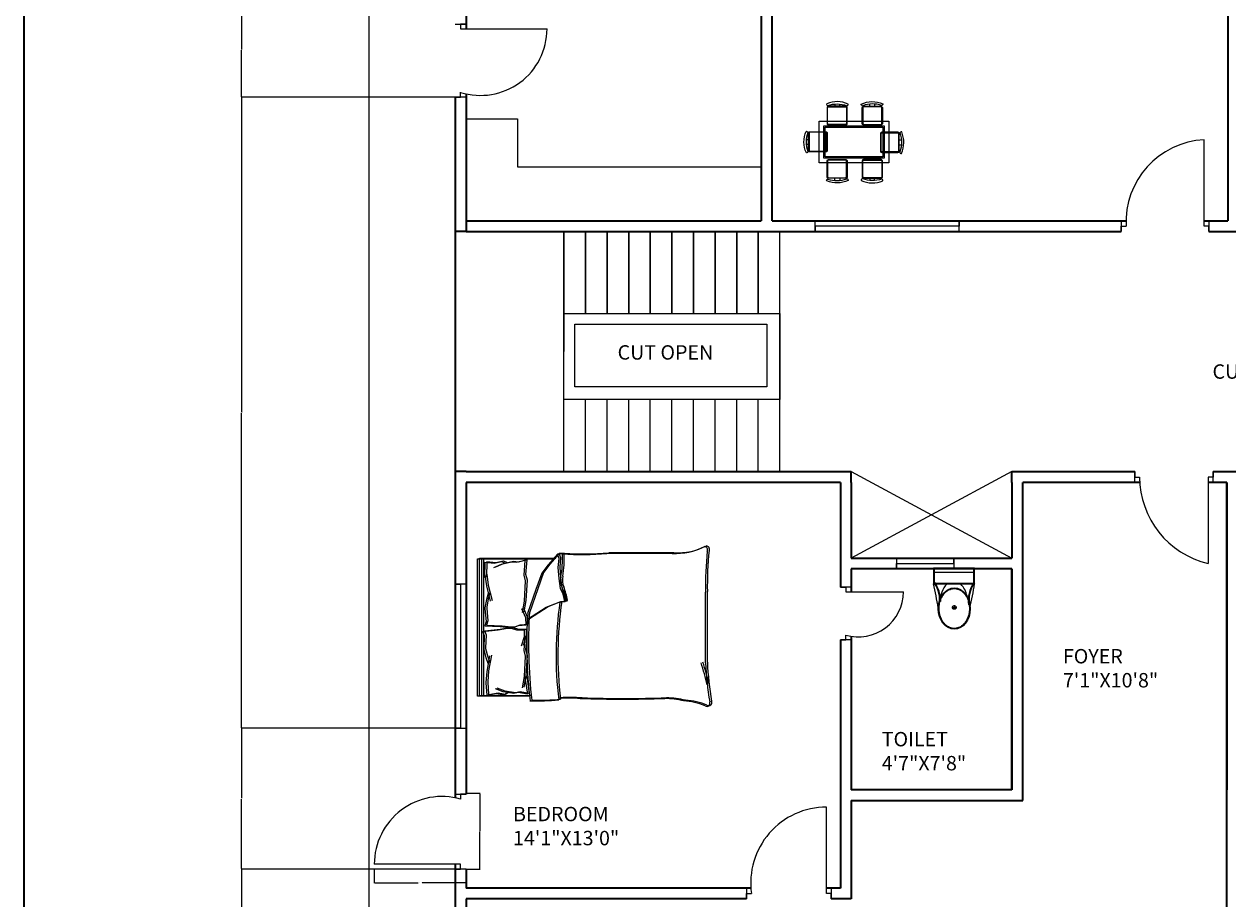
# Model space of a CAD drawing. Units: inches. Extents: x 1520 to 3401, y 1570 to 3432.
# Tile 4 of 15: x 1520 to 2022, y 2061 to 2425. Entities that reach past the tile are written whole.
import ezdxf

# ---------------------------------------------------------------- set-up
doc = ezdxf.new("R2010")
doc.units = ezdxf.units.IN
for name, color, linetype, lineweight in [('A-ANNO-DIMS', 2, 'Continuous', 18), ('A-ANNO-TTLB', 7, 'Continuous', 35), ('A-AREA-IDEN', 7, 'Continuous', 18), ('A-DOOR', 3, 'Continuous', 18), ('A-FLOR-CASE', 8, 'Continuous', 18), ('A-FLOR-EDGE', 7, 'Continuous', 25), ('A-FLOR-FIXT', 9, 'Continuous', 18), ('A-FLOR-OPEN', 8, 'Continuous', 13), ('A-FLOR-STRS', 2, 'Continuous', 18), ('A-FURN', 8, 'Continuous', 13), ('A-GLAZ', 4, 'Continuous', 18), ('A-WALL', 7, 'Continuous', 35)]:
    doc.layers.add(name, color=color, linetype=linetype, lineweight=lineweight)
doc.styles.get("Standard").update_dxf_attribs({"font": 'arial.ttf'})
doc.dimstyles.get("Standard").update_dxf_attribs({"dimtxt": 0.18, "dimasz": 0.18, "dimexe": 0.18, "dimexo": 0.0625, "dimgap": 0.09, "dimtad": 0, "dimtih": 1, "dimtoh": 1, "dimdec": 4, "dimzin": 0, "dimdsep": 46, "dimtxsty": 'Standard', "dimcen": 0.09, "dimadec": 0, "dimazin": 0, "dimtfac": 1, "dimtdec": 4, "dimtofl": 0, "dimtmove": 0, "dimatfit": 3, "dimfxl": 1, "dimtolj": 1, "dimtzin": 0, "dimarcsym": 0})

# ---------------------------------------------------------------- blocks, each defined once
blk = doc.blocks.new('A$C31115884')
for p, q in [((283, 498), (223, 498)), ((258, 466), (258, 523)), ((0, 200), (0, 0)), ((520, 200), (0, 200)), ((10, 190), (10, 10)), ((510, 190), (10, 190)), ((510, 10), (510, 190)), ((520, 0), (520, 200)), ((510, 54), (0, 54)), ((10, 10), (510, 10)), ((0, 0), (520, 0))]:
    blk.add_line(p, q)
blk.add_circle((256, 496), 23.6)
for centre, radius, start, end in [((2778, -205), 2807, 165.4549, 171.7133), ((-295, 403), 365, 324.2091, 9.3499), ((-295, 403), 375, 324.2091, 9.3499), ((806, 403), 365, 170.6501, 215.7909), ((3237, 905), 2807, 188.2867, 194.5451), ((384, 406), 293, 190.2774, 224.1564), ((139, 406), 293, 315.8436, 2.6563), ((806, 403), 375, 179.2036, 215.7909)]:
    blk.add_arc(centre, radius, start, end)
blk.add_ellipse((256, 510), major_axis=(0, -261), ratio=0.772727)
blk.add_open_spline([(256, 259), (263, 259), (270, 260), (288, 262), (299, 265), (320, 273), (330, 278), (350, 291), (360, 299), (378, 316), (386, 326), (402, 347), (409, 358), (421, 383), (427, 395), (436, 422), (440, 436), (445, 465), (447, 480), (448, 509), (448, 524), (445, 553), (443, 568), (436, 596), (432, 610), (422, 636), (416, 649), (402, 672), (395, 683), (379, 703), (370, 712), (351, 728), (341, 735), (321, 746), (310, 751), (289, 757), (278, 759), (256, 761), (245, 761), (223, 757), (212, 754), (191, 746), (181, 741), (161, 728), (151, 720), (133, 703), (125, 693), (110, 672), (103, 660), (90, 636), (85, 623), (76, 596), (72, 582), (67, 553), (66, 538), (64, 509), (65, 494), (68, 465), (70, 450), (77, 422), (81, 408), (91, 382), (97, 370), (111, 346), (118, 335), (135, 316), (144, 307), (162, 291), (172, 284), (193, 273), (203, 269), (225, 262), (236, 260), (250, 259), (253, 259), (256, 259)], degree=3, knots=[0, 0, 0, 0, 0.110105, 0.110105, 0.285049, 0.285049, 0.459994, 0.459994, 0.634938, 0.634938, 0.809882, 0.809882, 0.984827, 0.984827, 1.159771, 1.159771, 1.334715, 1.334715, 1.50966, 1.50966, 1.684604, 1.684604, 1.859549, 1.859549, 2.034493, 2.034493, 2.209437, 2.209437, 2.384382, 2.384382, 2.559326, 2.559326, 2.73427, 2.73427, 2.909215, 2.909215, 3.084159, 3.084159, 3.259103, 3.259103, 3.434048, 3.434048, 3.608992, 3.608992, 3.783936, 3.783936, 3.958881, 3.958881, 4.133825, 4.133825, 4.30877, 4.30877, 4.483714, 4.483714, 4.658658, 4.658658, 4.833603, 4.833603, 5.008547, 5.008547, 5.183491, 5.183491, 5.358436, 5.358436, 5.53338, 5.53338, 5.708324, 5.708324, 5.883269, 5.883269, 6.058213, 6.058213, 6.233158, 6.233158, 6.283185, 6.283185, 6.283185, 6.283185])
blk = doc.blocks.new('DOOR-SWING-36-09')
for p, q in [((34.55, 2.25), (34.55, 38.25)), ((0, 4.5), (0, 0)), ((0, 0), (0, 2.25)), ((0, 2.25), (2, 2.25)), ((36.55, 2.25), (34.55, 2.25)), ((36.55, 4.5), (36.55, 0)), ((36.55, 0), (36.55, 2.25))]:
    blk.add_line(p, q)
blk.add_arc((36.37, 3.88), 34.41, 93.0408, 182.7237)
blk = doc.blocks.new('DOOR-SWING-24-14')
for p, q in [((4.5, 21.95), (0, 21.95)), ((0, 21.95), (2.25, 21.95)), ((2.25, 21.95), (2.25, 19.95)), ((2.25, 19.95), (26.25, 19.95)), ((4.5, 0), (0, 0)), ((0, 0), (2.25, 0)), ((2.25, 0), (2.25, 2))]:
    blk.add_line(p, q)
blk.add_arc((7.54, 19.95), 18.71, 253.5847, 0)
blk = doc.blocks.new('DOOR-SWING-36-15')
for p, q in [((33.3, 2.25), (33.3, 38.25)), ((0, 4.5), (0, 0)), ((0, 0), (0, 2.25)), ((0, 2.25), (2, 2.25)), ((35.3, 2.25), (33.3, 2.25)), ((35.3, 4.5), (35.3, 0)), ((35.3, 0), (35.3, 2.25))]:
    blk.add_line(p, q)
blk.add_arc((33.3, 6.65), 31.6, 90, 187.995)
blk = doc.blocks.new('DOOR-SWING-36-17')
for p, q in [((0, 33.75), (0, 38.25)), ((0, 38.25), (0, 36)), ((0, 36), (2, 36)), ((32.63, 36), (30.63, 36)), ((30.63, 36), (30.63, 0)), ((32.63, 33.75), (32.63, 38.25)), ((32.63, 38.25), (32.63, 36))]:
    blk.add_line(p, q)
blk.add_arc((38.95, 36), 36.95, 180, 256.9796)
blk = doc.blocks.new('DOOR-SWING-36-24')
for p, q in [((0, 30.42), (4.5, 30.42)), ((4.5, 30.42), (2.25, 30.42)), ((2.25, 30.42), (2.25, 28.42)), ((2.25, 28.42), (38.25, 28.42)), ((4.5, 0), (0, 0)), ((0, 0), (2.25, 0)), ((2.25, 0), (2.25, 2))]:
    blk.add_line(p, q)
blk.add_arc((10.55, 28.42), 27.7, 252.5577, 0)
blk = doc.blocks.new('DOOR-SWING-36-25')
for p, q in [((33.75, 31.15), (38.25, 31.15)), ((38.25, 31.15), (36, 31.15)), ((36, 31.15), (36, 29.15)), ((36, 2), (0, 2)), ((38.25, 0), (33.75, 0)), ((33.75, 0), (36, 0)), ((36, 0), (36, 2))]:
    blk.add_line(p, q)
blk.add_arc((28.23, 2), 28.23, 74.0345, 180)
blk = doc.blocks.new('WIN-PLAN-24-01')
for p, q in [((0, 4.5), (0, 0)), ((0, 0), (0, 2.25)), ((0, 2.25), (24, 2.25)), ((24, 2.25), (24, 4.5)), ((24, 4.5), (24, 0))]:
    blk.add_line(p, q)
blk = doc.blocks.new('WIN-PLAN-60-02')
for p, q in [((4.5, 60), (0, 60)), ((0, 60), (2.25, 60)), ((2.25, 60), (2.25, 0)), ((4.5, 0), (0, 0)), ((2.25, 0), (4.5, 0))]:
    blk.add_line(p, q)
blk = doc.blocks.new('WIN-PLAN-60-03')
for p, q in [((0, 2.25), (0, 4.5)), ((0, 4.5), (0, 0)), ((60, 2.25), (0, 2.25)), ((60, 0), (60, 4.5)), ((60, 4.5), (60, 2.25))]:
    blk.add_line(p, q)
blk = doc.blocks.new('BED-DOUBLE')
for p, q in [((4.17, 75.93), (4.17, 97.64)), ((4.17, 97.64), (61.46, 97.64)), ((4.17, 95.8), (61.46, 95.8)), ((4.44, 75.16), (4.44, 96.87)), ((4.44, 96.87), (61.73, 96.87)), ((29.42, 94.7), (31.15, 95.4)), ((31.15, 95.4), (31.84, 88.98)), ((61.46, 97.64), (61.46, 65.74)), ((61.73, 96.87), (61.73, 64.97)), ((4.44, 95.03), (61.73, 95.03)), ((4.67, 93.64), (9.81, 94.03)), ((4.67, 93.66), (5.36, 89.85)), ((4.94, 92.9), (5.64, 89.08)), ((4.95, 92.87), (10.08, 93.27)), ((9.81, 94.03), (9.93, 94.01)), ((9.93, 94.01), (14.52, 93.66)), ((10.08, 93.27), (10.21, 93.24)), ((10.21, 93.24), (14.79, 92.9)), ((14.52, 93.66), (21.1, 92.45)), ((14.79, 92.9), (21.38, 91.68)), ((17.81, 93.14), (20.24, 94.01)), ((18.08, 92.38), (20.51, 93.24)), ((20.24, 94.01), (23.7, 94.88)), ((20.51, 93.24), (23.98, 94.11)), ((23.7, 94.88), (24.09, 94.88)), ((23.98, 94.11), (24.36, 94.11)), ((24.09, 94.88), (29.42, 94.7)), ((24.36, 94.11), (29.69, 93.94)), ((29.69, 93.94), (31.42, 94.63)), ((31.42, 94.63), (32.12, 88.22)), ((33.54, 94.65), (33.25, 88.21)), ((33.81, 93.88), (33.52, 87.44)), ((35.31, 94.07), (33.54, 94.65)), ((35.59, 93.3), (33.81, 93.88)), ((40.62, 94.57), (35.31, 94.07)), ((40.9, 93.81), (35.59, 93.3)), ((41.01, 94.6), (40.62, 94.57)), ((41.28, 93.83), (40.9, 93.81)), ((44.52, 93.95), (41.01, 94.6)), ((44.79, 93.18), (41.28, 93.83)), ((50.25, 93.96), (43.75, 92.34)), ((50.52, 93.19), (44.03, 91.57)), ((47, 93.23), (44.52, 93.95)), ((47.27, 92.47), (44.79, 93.18)), ((54.8, 94.59), (50.25, 93.96)), ((55.08, 93.82), (50.52, 93.19)), ((60.08, 94.57), (53.6, 94.69)), ((53.6, 94.69), (54.8, 94.59)), ((60.35, 93.81), (53.87, 93.92)), ((53.87, 93.92), (55.08, 93.82)), ((59.12, 87.74), (57.7, 90.95)), ((60.08, 94.57), (59.62, 90.72)), ((59.62, 90.72), (60.34, 87.64)), ((60.35, 93.81), (59.9, 89.96)), ((5.36, 89.85), (4.84, 86.73)), ((4.84, 86.73), (5.54, 85.52)), ((5.64, 89.08), (5.12, 85.96)), ((5.12, 85.96), (5.81, 84.75)), ((5.36, 82.57), (6.06, 86.9)), ((5.64, 81.8), (6.33, 86.14)), ((6.06, 86.9), (7.27, 90.2)), ((6.33, 86.14), (7.54, 89.43)), ((31.84, 88.98), (32.54, 85.17)), ((32.12, 88.22), (32.81, 84.4)), ((33.25, 88.21), (32.79, 84.36)), ((33.52, 87.44), (33.07, 83.59)), ((59.39, 86.97), (57.97, 90.18)), ((60.08, 83.46), (59.12, 87.74)), ((60.35, 82.69), (59.39, 86.97)), ((60.34, 87.64), (59.72, 86.39)), ((59.9, 89.96), (60.61, 86.88)), ((60.61, 86.88), (59.99, 85.62)), ((5.02, 76.85), (5.71, 80.66)), ((5.71, 80.66), (5.36, 82.57)), ((5.98, 79.9), (5.64, 81.8)), ((32.54, 83.61), (31.84, 81.36)), ((31.84, 81.36), (31.84, 78.14)), ((32.81, 82.84), (32.12, 80.59)), ((32.12, 80.59), (32.12, 77.37)), ((32.54, 85.17), (32.54, 83.61)), ((32.79, 84.36), (32.89, 82.8)), ((32.81, 84.4), (32.81, 82.84)), ((32.89, 82.8), (33.72, 80.59)), ((33.07, 83.59), (33.17, 82.03)), ((33.17, 82.03), (34, 79.83)), ((33.72, 80.59), (33.93, 77.39)), ((59.85, 81.53), (60.08, 83.46)), ((60.78, 77.77), (59.85, 81.53)), ((60.12, 80.77), (60.35, 82.69)), ((61.05, 77), (60.12, 80.77)), ((11.13, 77.72), (5.02, 76.85)), ((5.29, 76.08), (5.98, 79.9)), ((11.4, 76.95), (5.29, 76.08)), ((7.65, 78.9), (12.48, 78.1)), ((7.92, 78.14), (12.76, 77.34)), ((12.48, 78.1), (11.13, 77.72)), ((12.76, 77.34), (11.4, 76.95)), ((12.48, 78.1), (20.89, 77.59)), ((12.76, 77.34), (21.16, 76.82)), ((20.89, 77.59), (23.24, 78.25)), ((21.16, 76.82), (23.51, 77.49)), ((23.24, 78.25), (29.39, 77.77)), ((23.51, 77.49), (29.67, 77)), ((28.9, 78.14), (25.13, 79.45)), ((29.17, 77.37), (25.4, 78.68)), ((31.84, 78.14), (28.9, 78.14)), ((32.12, 77.37), (29.17, 77.37)), ((33.93, 77.39), (36.87, 77.57)), ((34, 79.83), (34.2, 76.62)), ((34.2, 76.62), (37.14, 76.8)), ((36.28, 76.8), (41.3, 69.01)), ((36.55, 76.03), (41.57, 68.25)), ((36.87, 77.57), (40.55, 79.11)), ((37.14, 76.8), (40.82, 78.34)), ((48.73, 73.28), (38.73, 76.8)), ((49, 72.52), (39, 76.03)), ((39.04, 78.9), (43.87, 78.1)), ((39.31, 78.14), (44.15, 77.34)), ((43.87, 78.1), (52.28, 77.59)), ((44.15, 77.34), (52.55, 76.82)), ((52.28, 77.59), (54.63, 78.25)), ((52.55, 76.82), (54.9, 77.49)), ((54.63, 78.25), (60.78, 77.77)), ((54.9, 77.49), (61.05, 77)), ((55.41, 70.87), (48.73, 73.28)), ((55.69, 70.1), (49, 72.52)), ((58.94, 68.27), (55.41, 70.87)), ((41.3, 69.01), (43.34, 63.63)), ((41.57, 68.25), (43.62, 62.87)), ((59.21, 67.51), (55.69, 70.1)), ((63.38, 64.38), (58.94, 68.27)), ((63.66, 63.61), (59.21, 67.51)), ((43.34, 63.63), (43.71, 61.22)), ((43.62, 62.87), (43.99, 60.45)), ((43.71, 61.22), (46.68, 61.96)), ((43.99, 60.45), (46.96, 61.2)), ((46.68, 61.96), (49.1, 63.08)), ((46.96, 61.2), (49.37, 62.31)), ((49.1, 63.08), (53.18, 63.63)), ((49.37, 62.31), (53.46, 62.87)), ((53.18, 63.63), (57.82, 64)), ((53.46, 62.87), (58.1, 63.24)), ((57.82, 64), (61.54, 63.63)), ((58.1, 63.24), (61.81, 62.87)), ((61.54, 63.63), (63.38, 64.38)), ((61.81, 62.87), (63.66, 63.61)), ((63.48, 62.28), (63.38, 64.38, 4.64)), ((63.75, 61.52), (63.66, 63.61, 4.64)), ((18.06, 2.64), (47.57, 2.64)), ((18.33, 1.87), (47.84, 1.87))]:
    blk.add_line(p, q)
for centre, radius, start, end in [((102.1, 73.55), 99.87, 178.7218, 185.604), ((25.61, -120.62), 197.77, 86.0865, 96.7821), ((25.88, -121.38), 197.77, 86.0865, 96.7821), ((102.37, 72.78), 99.87, 178.7218, 185.604), ((21.29, -89.76), 154.68, 81.7845, 96.9006), ((21.56, -90.53), 154.68, 81.7845, 96.9006), ((-200.58, 60.27), 203.94, 358.4762, 1.0082), ((-200.3, 59.5), 203.94, 358.4762, 1.0082), ((43.92, 61.15), 0.221, 160.2464, 271.1377), ((37.35, 95.86), 35.55, 280.6617, 289.8806), ((44.2, 60.38), 0.221, 160.2464, 271.1377), ((37.62, 95.1), 35.55, 280.6617, 289.8806), ((52.44, 55.6), 7.46, 78.6608, 113.7384), ((52.72, 54.83), 7.46, 78.6608, 113.7384), ((61.53, 105.62), 43.38, 259.8763, 272.5657), ((61.81, 104.85), 43.38, 259.8763, 272.5657), ((218.51, 54.1), 155.25, 176.9791, 183.8365), ((218.79, 53.34), 155.25, 176.9791, 183.8365), ((581.23, 36.96), 578.22, 178.22771, 181.71854), ((581.51, 36.19), 578.22, 178.22771, 181.71854), ((-5405.34, 16.33), 5469.02, 0.00217, 0.28689), ((-5405.07, 15.56), 5469.02, 0.00217, 0.28689), ((-32.25, 20.29), 35.53, 346.0648, 358.9113), ((-31.97, 19.53), 35.53, 346.0648, 358.9113), ((91.3, 15.32), 27.65, 177.4714, 206.4681), ((91.58, 14.55), 27.65, 177.4714, 206.4681), ((-25.97, 13.39), 28.25, 337.9751, 356.652), ((-25.69, 12.62), 28.25, 337.9751, 356.652), ((1.3, 2.07), 1.31, 146.1736, 293.4781), ((1.58, 1.3), 1.31, 146.1736, 293.4781), ((25.69, -143.14), 145.97, 92.9958, 99.4091), ((25.96, -143.9), 145.97, 92.9958, 99.4091), ((-20.65, 126.07), 127.63, 283.3832, 287.7053), ((-20.37, 125.3), 127.63, 283.3832, 287.7053), ((49.34, -156.85), 159.5, 84.4998, 90.6351), ((49.61, -157.62), 159.5, 84.4998, 90.6351), ((65.23, 3.08), 1.32, 242.6588, 356.02), ((65.5, 2.32), 1.32, 242.6588, 356.02)]:
    blk.add_arc(centre, radius, start, end)
blk = doc.blocks.new('KITCHEN-COUNTER-04')
for p, q in [((0, 19.94), (21.46, 19.94)), ((21.46, 19.94), (21.46, 0)), ((21.46, 0), (123, 0)), ((123, 0), (123, 0))]:
    blk.add_line(p, q)
blk = doc.blocks.new('DINING-SET-6-SEAT')
for points in [[(9.94, 32.23, -0.175809), (17.84, 32.17, 0.578392), (18.44, 32.83, 0.214524), (9.52, 32.95, 0.552014), (9.94, 32.23, -0.065079)], [(17.51, 31.92), (10.17, 31.92, 0.414214), (9.66, 31.4), (9.66, 24.66, 0.414214), (10.17, 24.14), (17.51, 24.14, 0.414214), (18.02, 24.66), (18.02, 31.4, 0.414214), (17.51, 31.92)], [(14.93, 31.92), (14.93, 32.84, -0.064759)], [(24.5, 32.17, -0.578392), (23.9, 32.83, -0.214524), (32.82, 32.95, -0.552014), (32.4, 32.23, 0.175809), (24.5, 32.17)], [(32.17, 31.92, -0.414214), (32.68, 31.4), (32.68, 24.66, -0.414214), (32.17, 24.14), (24.83, 24.14, -0.414214), (24.32, 24.66), (24.32, 31.4, -0.414214), (24.83, 31.92), (32.17, 31.92)], [(27.41, 31.92), (27.41, 32.84, 0.064759)], [(1.67, 13.15, -0.578392), (1.02, 12.55, -0.214524), (0.9, 21.47, -0.552014), (1.61, 21.05, 0.175809), (1.67, 13.15)], [(1.93, 20.82, -0.414214), (2.45, 21.33), (9.19, 21.33, -0.414214), (9.7, 20.82), (9.7, 13.49, -0.414214), (9.19, 12.97), (2.45, 12.97, -0.414214), (1.93, 13.49), (1.93, 20.82)], [(39.71, 20.57, 0.414214), (39.19, 21.08), (32.45, 21.08, 0.414214), (31.94, 20.57), (31.94, 13.23, 0.414214), (32.45, 12.72), (39.19, 12.72, 0.414214), (39.71, 13.23), (39.71, 20.57)], [(40.02, 20.8, -0.175809), (39.96, 12.9, 0.578392), (40.62, 12.3, 0.214524), (40.74, 21.22, 0.552014), (40.02, 20.8, -0.065079)], [(1.93, 16.06), (1, 16.06, 0.064759)], [(39.71, 15.81), (40.63, 15.81, -0.064759)], [(17.51, 1.93), (10.17, 1.93, -0.414214), (9.66, 2.45), (9.66, 9.19, -0.414214), (10.17, 9.7), (17.51, 9.7, -0.414214), (18.02, 9.19), (18.02, 2.45, -0.414214), (17.51, 1.93)], [(32.17, 1.93, 0.414214), (32.68, 2.45), (32.68, 9.19, 0.414214), (32.17, 9.7), (24.83, 9.7, 0.414214), (24.32, 9.19), (24.32, 2.45, 0.414214), (24.83, 1.93), (32.17, 1.93)], [(17.84, 1.67, -0.578392), (18.44, 1.02, -0.214524), (9.52, 0.9, -0.552014), (9.94, 1.61, 0.175809), (17.84, 1.67)], [(14.93, 1.93), (14.93, 1, 0.064759)], [(32.4, 1.61, -0.175809), (24.5, 1.67, 0.578392), (23.9, 1.02, 0.214524), (32.82, 0.9, 0.552014), (32.4, 1.61, -0.065079)], [(27.41, 1.93), (27.41, 1, -0.064759)]]:
    blk.add_lwpolyline(points, format="xyb")
for points in [[(10.18, 31.68), (17.28, 31.68, -0.414214), (17.79, 31.17), (17.79, 24.89, -0.414214), (17.28, 24.37), (10.18, 24.37, -0.512069), (9.89, 24.89), (9.89, 31.17, -0.512069)], [(32.16, 31.68), (25.06, 31.68, 0.414214), (24.55, 31.17), (24.55, 24.89, 0.414214), (25.06, 24.37), (32.16, 24.37, 0.512069), (32.45, 24.89), (32.45, 31.17, 0.512069)], [(2.16, 20.82), (2.16, 13.72, 0.414214), (2.68, 13.2), (8.96, 13.2, 0.414214), (9.47, 13.72), (9.47, 20.82, 0.512069), (8.96, 21.1), (2.68, 21.1, 0.512069)], [(39.48, 20.57), (39.48, 13.47, -0.414214), (38.96, 12.95), (32.68, 12.95, -0.414214), (32.17, 13.47), (32.17, 20.57, -0.512069), (32.68, 20.85), (38.96, 20.85, -0.512069)], [(10.18, 2.16), (17.28, 2.16, 0.414214), (17.79, 2.68), (17.79, 8.96, 0.414214), (17.28, 9.47), (10.18, 9.47, 0.512069), (9.89, 8.96), (9.89, 2.68, 0.512069)], [(32.16, 2.16), (25.06, 2.16, -0.414214), (24.55, 2.68), (24.55, 8.96, -0.414214), (25.06, 9.47), (32.16, 9.47, -0.512069), (32.45, 8.96), (32.45, 2.68, -0.512069)]]:
    blk.add_lwpolyline(points, format="xyb", close=True)
for points in [[(12.88, 32.86), (12.88, 31.92)], [(29.46, 32.86), (29.46, 31.92)], [(0.99, 18.12), (1.93, 18.12)], [(40.65, 17.86), (39.71, 17.86)], [(12.88, 0.99), (12.88, 1.93)], [(29.46, 0.99), (29.46, 1.93)]]:
    blk.add_lwpolyline(points)
for points in [[(6.35, 25.72), (35.36, 25.72), (35.36, 8.31), (6.35, 8.31)], [(8.29, 23.79), (33.43, 23.79), (33.43, 10.25), (8.29, 10.25)], [(8.87, 23.21), (32.85, 23.21), (32.85, 10.83), (8.87, 10.83)]]:
    blk.add_lwpolyline(points, close=True)
blk = doc.blocks.new('*D129')
at = {"layer": 'A-ANNO-DIMS', "color": 0, "lineweight": -2, "transparency": 16777216}
for p, q in [((1665.86, 2073.06), (1665.86, 2067.2)), ((1704.11, 2073.06), (1704.11, 2067.2)), ((1666.04, 2067.38), (1684.2, 2067.38)), ((1703.93, 2067.38), (1685.78, 2067.38))]:
    blk.add_line(p, q, dxfattribs=at)
at = {"layer": 'A-ANNO-DIMS', "color": 0, "transparency": 16777216}
for points in [[(1666.04, 2067.41), (1666.04, 2067.35), (1665.86, 2067.38)], [(1703.93, 2067.41), (1703.93, 2067.35), (1704.11, 2067.38)]]:
    blk.add_solid(points, dxfattribs=at)
at = {"layer": 'Defpoints', "color": 0, "transparency": 16777216}
for p in [(1665.86, 2073.12), (1704.11, 2073.12), (1704.11, 2067.38)]:
    blk.add_point(p, dxfattribs=at)
at = {"layer": 'A-ANNO-DIMS', "color": 0, "transparency": 16777216, "insert": (1684.99, 2067.38), "char_height": 0.18, "attachment_point": 5}
blk.add_mtext('\\A1;D25 38 TYP.', dxfattribs=at)
blk = doc.blocks.new('*D130')
at = {"layer": 'A-ANNO-DIMS', "color": 0, "lineweight": -2, "transparency": 16777216}
for p, q in [((1704.18, 2104.7), (1710.03, 2104.7)), ((1709.85, 2104.52), (1709.85, 2089.09)), ((1709.85, 2073.3), (1709.85, 2088.73)), ((1704.18, 2073.12), (1710.03, 2073.12))]:
    blk.add_line(p, q, dxfattribs=at)
at = {"layer": 'A-ANNO-DIMS', "color": 0, "transparency": 16777216}
for points in [[(1709.82, 2104.52), (1709.88, 2104.52), (1709.85, 2104.7)], [(1709.82, 2073.3), (1709.88, 2073.3), (1709.85, 2073.12)]]:
    blk.add_solid(points, dxfattribs=at)
at = {"layer": 'Defpoints', "color": 0, "transparency": 16777216}
for p in [(1704.11, 2104.7), (1709.85, 2104.7), (1704.11, 2073.12)]:
    blk.add_point(p, dxfattribs=at)
at = {"layer": 'A-ANNO-DIMS', "color": 0, "transparency": 16777216, "insert": (1709.85, 2088.91), "char_height": 0.18, "attachment_point": 5}
blk.add_mtext('\\A1;32 TYP.', dxfattribs=at)
blk = doc.blocks.new('*D187')
at = {"layer": 'A-ANNO-DIMS', "color": 0, "lineweight": -2, "transparency": 16777216}
for p, q in [((1699.55, 2073.12), (1610.33, 2073.12)), ((1610.51, 2072.94), (1610.51, 2023.24)), ((1610.51, 1973.18), (1610.51, 2022.88)), ((1699.55, 1973), (1610.33, 1973))]:
    blk.add_line(p, q, dxfattribs=at)
at = {"layer": 'A-ANNO-DIMS', "color": 0, "transparency": 16777216}
for points in [[(1610.48, 2072.94), (1610.54, 2072.94), (1610.51, 2073.12)], [(1610.48, 1973.18), (1610.54, 1973.18), (1610.51, 1973)]]:
    blk.add_solid(points, dxfattribs=at)
at = {"layer": 'Defpoints', "color": 0, "transparency": 16777216}
for p in [(1610.51, 2073.12), (1699.61, 2073.12), (1699.61, 1973)]:
    blk.add_point(p, dxfattribs=at)
at = {"layer": 'A-ANNO-DIMS', "color": 0, "transparency": 16777216, "insert": (1610.51, 2023.06), "char_height": 0.18, "attachment_point": 5}
blk.add_mtext('\\A1;100.12', dxfattribs=at)
blk = doc.blocks.new('*D188')
at = {"layer": 'A-ANNO-DIMS', "color": 0, "lineweight": -2, "transparency": 16777216}
for p, q in [((1699.55, 2131.83), (1610.33, 2131.83)), ((1610.51, 2131.65), (1610.51, 2102.66)), ((1610.51, 2073.3), (1610.51, 2102.29)), ((1699.55, 2073.12), (1610.33, 2073.12))]:
    blk.add_line(p, q, dxfattribs=at)
at = {"layer": 'A-ANNO-DIMS', "color": 0, "transparency": 16777216}
for points in [[(1610.48, 2131.65), (1610.54, 2131.65), (1610.51, 2131.83)], [(1610.48, 2073.3), (1610.54, 2073.3), (1610.51, 2073.12)]]:
    blk.add_solid(points, dxfattribs=at)
at = {"layer": 'Defpoints', "color": 0, "transparency": 16777216}
for p in [(1610.51, 2131.83), (1699.61, 2131.83), (1699.61, 2073.12)]:
    blk.add_point(p, dxfattribs=at)
at = {"layer": 'A-ANNO-DIMS', "color": 0, "transparency": 16777216, "insert": (1610.51, 2102.48), "char_height": 0.18, "attachment_point": 5}
blk.add_mtext('\\A1;58.71', dxfattribs=at)
blk = doc.blocks.new('*D189')
at = {"layer": 'A-ANNO-DIMS', "color": 0, "lineweight": -2, "transparency": 16777216}
for p, q in [((1699.55, 2394.67), (1610.33, 2394.67)), ((1610.51, 2394.49), (1610.51, 2263.44)), ((1610.51, 2132.01), (1610.51, 2263.07)), ((1699.55, 2131.83), (1610.33, 2131.83))]:
    blk.add_line(p, q, dxfattribs=at)
at = {"layer": 'A-ANNO-DIMS', "color": 0, "transparency": 16777216}
for points in [[(1610.48, 2394.49), (1610.54, 2394.49), (1610.51, 2394.67)], [(1610.48, 2132.01), (1610.54, 2132.01), (1610.51, 2131.83)]]:
    blk.add_solid(points, dxfattribs=at)
at = {"layer": 'Defpoints', "color": 0, "transparency": 16777216}
for p in [(1610.51, 2394.67), (1699.61, 2394.67), (1699.61, 2131.83)]:
    blk.add_point(p, dxfattribs=at)
at = {"layer": 'A-ANNO-DIMS', "color": 0, "transparency": 16777216, "insert": (1610.51, 2263.25), "char_height": 0.18, "attachment_point": 5}
blk.add_mtext('\\A1;262.84', dxfattribs=at)
blk = doc.blocks.new('*D190')
at = {"layer": 'A-ANNO-DIMS', "color": 0, "lineweight": -2, "transparency": 16777216}
for p, q in [((1699.55, 2434.03), (1610.33, 2434.03)), ((1610.51, 2433.85), (1610.51, 2414.53)), ((1610.51, 2394.85), (1610.51, 2414.17)), ((1699.55, 2394.67), (1610.33, 2394.67))]:
    blk.add_line(p, q, dxfattribs=at)
at = {"layer": 'A-ANNO-DIMS', "color": 0, "transparency": 16777216}
for points in [[(1610.48, 2433.85), (1610.54, 2433.85), (1610.51, 2434.03)], [(1610.48, 2394.85), (1610.54, 2394.85), (1610.51, 2394.67)]]:
    blk.add_solid(points, dxfattribs=at)
at = {"layer": 'Defpoints', "color": 0, "transparency": 16777216}
for p in [(1610.51, 2434.03), (1699.61, 2434.03), (1699.61, 2394.67)]:
    blk.add_point(p, dxfattribs=at)
at = {"layer": 'A-ANNO-DIMS', "color": 0, "transparency": 16777216, "insert": (1610.51, 2414.35), "char_height": 0.18, "attachment_point": 5}
blk.add_mtext('\\A1;39.36', dxfattribs=at)

msp = doc.modelspace()

# ---------------------------------------------------------------- linework, layer by layer
at = {"layer": 'A-ANNO-TTLB'}
msp.add_lwpolyline([(1519.9253, 3431.7421), (3400.8761, 3431.7421), (3400.8761, 1570.3458), (1519.9253, 1570.3458)], close=True, dxfattribs=at)
at = {"layer": 'A-AREA-IDEN'}
msp.add_lwpolyline([(1749.4596, 2300.0971), (1829.5099, 2300.0971), (1829.5099, 2274.0317), (1749.4596, 2274.0317)], close=True, dxfattribs=at)
at = {"layer": 'A-FLOR-EDGE'}
msp.add_line((1663.6128, 2733.1786), (1663.6128, 1791.6786), dxfattribs=at)
at = {"layer": 'A-FLOR-OPEN'}
for p, q in [((1931.6128, 2238.6786), (1864.6128, 2202.6786)), ((1864.6128, 2238.6786), (1931.6128, 2202.6786))]:
    msp.add_line(p, q, dxfattribs=at)
at = {"layer": 'A-FLOR-STRS'}
for p, q in [((1744.8908, 2238.6786), (1744.8908, 2338.6786)), ((1744.8908, 2338.6786), (1744.8908, 2288.6786)), ((1753.8908, 2338.6786), (1753.8908, 2304.5362)), ((1753.8908, 2304.5362), (1753.8908, 2338.6786)), ((1762.8908, 2338.6786), (1762.8908, 2304.5362)), ((1762.8908, 2304.5362), (1762.8908, 2338.6786)), ((1771.8908, 2338.6786), (1771.8908, 2304.5362)), ((1771.8908, 2304.5362), (1771.8908, 2338.6786)), ((1780.8908, 2338.6786), (1780.8908, 2304.5362)), ((1780.8908, 2304.5362), (1780.8908, 2338.6786)), ((1789.8908, 2338.6786), (1789.8908, 2304.5362)), ((1789.8908, 2304.5362), (1789.8908, 2338.6786)), ((1798.8908, 2338.6786), (1798.8908, 2304.5362)), ((1798.8908, 2304.5362), (1798.8908, 2338.6786)), ((1807.8908, 2338.6786), (1807.8908, 2304.5362)), ((1807.8908, 2304.5362), (1807.8908, 2338.6786)), ((1816.8908, 2338.6786), (1816.8908, 2304.5362)), ((1816.8908, 2304.5362), (1816.8908, 2338.6786)), ((1825.8908, 2338.6786), (1825.8908, 2304.5362)), ((1825.8908, 2304.5362), (1825.8908, 2338.6786)), ((1834.8908, 2238.6786), (1834.8908, 2338.6786)), ((1744.8908, 2304.5362), (1834.8908, 2304.5362)), ((1834.8908, 2304.5362), (1834.8908, 2268.682)), ((1834.8908, 2268.682), (1744.8908, 2268.682)), ((1753.8908, 2238.6786), (1753.8908, 2268.682)), ((1762.8908, 2238.6786), (1762.8908, 2268.682)), ((1771.8908, 2238.6786), (1771.8908, 2268.682)), ((1780.8908, 2238.6786), (1780.8908, 2268.682)), ((1789.8908, 2238.6786), (1789.8908, 2268.682)), ((1798.8908, 2238.6786), (1798.8908, 2268.682)), ((1807.8908, 2238.6786), (1807.8908, 2268.682)), ((1816.8908, 2238.6786), (1816.8908, 2268.682)), ((1825.8908, 2238.6786), (1825.8908, 2268.682))]:
    msp.add_line(p, q, dxfattribs=at)
at = {"layer": 'A-WALL'}
for p, q in [((2021.6128, 2558.1786), (2021.6128, 2343.1786)), ((1704.1128, 2508.6786), (1704.1128, 2423.0977)), ((1827.1128, 2447.697), (1827.1128, 2343.1786)), ((1831.6128, 2343.1786), (1831.6128, 2447.697)), ((1699.6128, 2394.6735), (1699.6128, 2102.8094)), ((1699.6128, 2394.6735), (1699.6128, 2102.8094)), ((1704.1128, 2396.0692), (1704.1128, 2338.6786)), ((1704.1128, 2343.1786), (1827.1128, 2343.1786)), ((1831.6128, 2343.1786), (1979.1306, 2343.1786)), ((2011.7128, 2343.1786), (2021.6128, 2343.1786)), ((1704.1128, 2338.6786), (1699.6128, 2338.6786)), ((1704.1128, 2338.6786), (1977.164, 2338.6786)), ((2013.7128, 2338.6786), (2163.0531, 2338.6786)), ((1704.1128, 2238.6786), (1699.6128, 2238.6786)), ((1704.1128, 2238.6786), (1864.6128, 2238.6786)), ((1864.6128, 2234.1786), (1864.6128, 2238.6786)), ((1931.6128, 2234.1786), (1931.6128, 2238.6786)), ((1931.6128, 2238.6786), (1982.8022, 2238.6786)), ((2015.4274, 2238.6786), (2227.7862, 2238.6786)), ((1704.1128, 2234.1786), (1704.1128, 2104.2644)), ((1860.1128, 2234.1786), (1704.1128, 2234.1786)), ((1860.1128, 2234.1786), (1860.1128, 2190.5406)), ((1864.6128, 2234.1786), (1864.6128, 2202.6786)), ((1931.6128, 2234.1786), (1931.6128, 2202.6786)), ((1936.1128, 2106.1786), (1936.1128, 2234.1786)), ((1984.8707, 2234.1786), (1936.1128, 2234.1786)), ((2021.1128, 2234.1786), (2013.4274, 2234.1786)), ((2021.1128, 1923.6786), (2021.1128, 2234.1786)), ((2021.1128, 2234.1786), (2021.1128, 2106.1786)), ((1864.6128, 2202.6786), (1931.6128, 2202.6786)), ((1931.6128, 2198.1786), (1864.6128, 2198.1786)), ((1864.6128, 2198.1786), (1864.6128, 2188.5406)), ((1931.6128, 2106.1786), (1931.6128, 2198.1786)), ((1931.6128, 2198.1786), (1931.6128, 2106.1786)), ((1860.1128, 2168.5913), (1860.1128, 2065.1786)), ((1864.6128, 2170.0769), (1864.6128, 2106.1786)), ((1931.6128, 2106.1786), (1864.6128, 2106.1786)), ((1936.1128, 2101.6786), (1936.1128, 2106.1786)), ((1864.6128, 2101.6786), (1936.1128, 2101.6786)), ((1864.6128, 2101.6786), (1864.6128, 2060.6786)), ((1699.6128, 2075.1195), (1699.6128, 1924.1968)), ((1699.6128, 2075.1195), (1699.6128, 1924.1968)), ((1704.1128, 2073.1195), (1704.1128, 2065.1786)), ((1822.8049, 2065.1786), (1704.1128, 2065.1786)), ((1860.1128, 2065.1786), (1854.3362, 2065.1786)), ((1704.1128, 2060.6786), (1704.1128, 1922.1968)), ((1821.0391, 2060.6786), (1704.1128, 2060.6786)), ((1864.6128, 2060.6786), (1856.3362, 2060.6786))]:
    msp.add_line(p, q, dxfattribs=at)

# ---------------------------------------------------------------- block references
at = {"layer": 'A-DOOR'}
for name, p in [('DOOR-SWING-36-24', (1699.613, 2394.673)), ('DOOR-SWING-36-09', (1977.164, 2338.679)), ('DOOR-SWING-36-17', (1982.802, 2200.429)), ('DOOR-SWING-24-14', (1860.113, 2168.591)), ('DOOR-SWING-36-25', (1665.863, 2073.119)), ('DOOR-SWING-36-15', (1821.039, 2060.679))]:
    msp.add_blockref(name, p, dxfattribs=at)
at = {"layer": 'A-FLOR-CASE'}
msp.add_blockref('KITCHEN-COUNTER-04', (1704.113, 2365.63), dxfattribs=at)
at = {"layer": 'A-FLOR-FIXT', "xscale": 0.0330640103915726, "yscale": 0.0330640103915726, "zscale": 0.0330640103915726, "rotation": 180}
msp.add_blockref('A$C31115884', (1916.043, 2198.5093), dxfattribs=at)
at = {"layer": 'A-FURN'}
msp.add_blockref('DINING-SET-6-SEAT', (1844.9134, 2358.9365), dxfattribs=at)
at = {"layer": 'A-FURN', "rotation": 90.00000000000003}
msp.add_blockref('BED-DOUBLE', (1806.5356, 2140.901), dxfattribs=at)
at = {"layer": 'A-GLAZ'}
for name, p, rotation in [('WIN-PLAN-60-02', (1849.5837, 2343.1785), 270), ('WIN-PLAN-60-03', (1704.1125, 2131.8338), 90)]:
    msp.add_blockref(name, p, dxfattribs=dict(at, rotation=rotation))
msp.add_blockref('WIN-PLAN-24-01', (1883.446, 2198.179), dxfattribs=at)

# ---------------------------------------------------------------- texts
at = {"layer": 'A-AREA-IDEN', "char_height": 6, "attachment_point": 1}
for s, width, insert in [('CUT OPEN', 105.215373, (1767.2687, 2291.3327)), ('CUT OPEN', 203.592059, (2015.1778, 2283.3623)), ('FOYER\\P7\'1"X10\'8"', 143.014964, (1952.8429, 2164.7771)), ('TOILET\\P4\'7"X7\'8"', 112.972634, (1877.3618, 2130.2221)), ('BEDROOM\\P14\'1"X13\'0"', 115.529743, (1723.6935, 2099.0322))]:
    msp.add_mtext_dynamic_manual_height_columns(s, width=width, gutter_width=12.5, heights=[0], dxfattribs=dict(at, insert=insert))

# ---------------------------------------------------------------- dimensions: what is measured, and where the dimension line sits
at = {"layer": 'A-ANNO-DIMS'}
for base, p1, p2, picture, middle in [((1610.5128, 2434.0307), (1699.6128, 2394.6735), (1699.6128, 2434.0307), '*D190', (1610.5128, 2414.3521)), ((1610.5128, 2394.6735), (1699.6128, 2131.8339), (1699.6128, 2394.6735), '*D189', (1610.5128, 2263.2537)), ((1610.5128, 2131.8339), (1699.6128, 2073.1195), (1699.6128, 2131.8339), '*D188', (1610.5128, 2102.4767)), ((1610.5128, 2073.1195), (1699.6128, 1973.0015), (1699.6128, 2073.1195), '*D187', (1610.5128, 2023.0605))]:
    dim = msp.add_linear_dim(base=base, p1=p1, p2=p2, angle=90, dimstyle='Standard', override={"dimdec": 2, "dimlfac": 1, "dimrnd": 0, "dimzin": 0, "dimdsep": 46, "dimlunit": 2}, dxfattribs=at)
    dim.commit()
    dim.dimension.update_dxf_attribs({"geometry": picture, "text_midpoint": middle})
dim = msp.add_linear_dim(base=(1709.8503, 2104.7018), p1=(1704.1128, 2073.1195), p2=(1704.1128, 2104.7018), angle=90, text='<> TYP.', dimstyle='Standard', override={"dimdec": 0, "dimlfac": 1, "dimrnd": 0, "dimzin": 0, "dimdsep": 46, "dimlunit": 2}, dxfattribs=at)
dim.commit()
dim.dimension.update_dxf_attribs({"geometry": '*D130', "text_midpoint": (1709.8503, 2088.9107)})
dim = msp.add_linear_dim(base=(1704.1128, 2067.382), p1=(1665.8628, 2073.1195), p2=(1704.1128, 2073.1195), text='D25 <> TYP.', dimstyle='Standard', override={"dimdec": 0, "dimlfac": 1, "dimrnd": 0, "dimzin": 0, "dimdsep": 46, "dimlunit": 2}, dxfattribs=at)
dim.commit()
dim.dimension.update_dxf_attribs({"geometry": '*D129', "text_midpoint": (1684.9878, 2067.382)})

doc.saveas('drawing.dxf')
